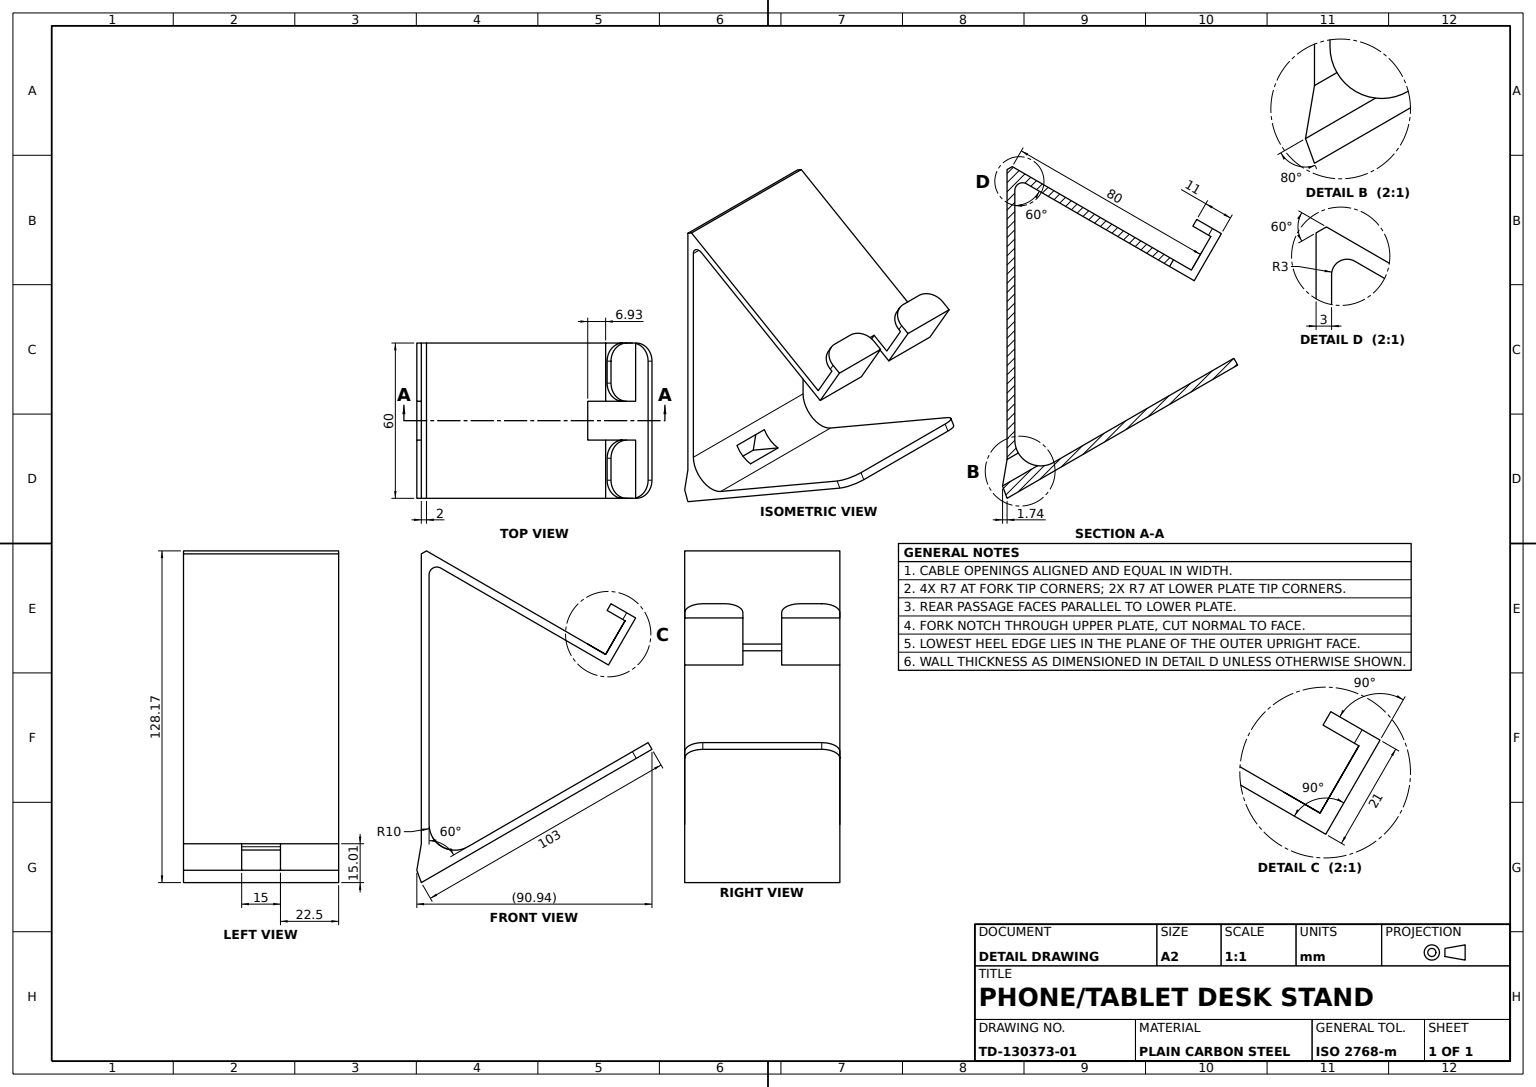
SolidWorks part; units mm, degrees
material "Plain Carbon Steel"
ref_plane "Front Plane" through (0, 0, 0) normal (0, 0, 1) x (1, 0, 0)
ref_plane "Top Plane" through (0, 0, 0) normal (0, 1, 0) x (1, 0, 0)
ref_plane "Right Plane" through (0, 0, 0) normal (1, 0, 0) x (0, 0, -1)
sketch "Stand Profile Sketch" plane through (0, 0, 0) normal (0, 0, 1) x (1, 0, 0)
  line L0 (0, 0) -> (80.4833, 0)
  line L1 (89.1436, 15) -> (40.9348, 98.5)
  line L2 (35.7387, 98.5) -> (-1.7199, 33.6199)
  line L3 (-1.7199, 33.6199) -> (-19.9064, 44.1199)
  line L4 (-19.9064, 44.1199) -> (-14.4064, 53.6462)
  line L5 (0, -3) -> (103, -3)
  line L6 (95.4944, 10) -> (39.4915, 107)
  line L7 (37.1821, 107) -> (-2.8179, 37.718)
  line L8 (-2.8179, 37.718) -> (-15.8083, 45.218)
  line L9 (-15.8083, 45.218) -> (-11.8083, 52.1462)
  line L10 (-14.4064, 53.6462) -> (-11.8083, 52.1462)
  line L11 (0, 0) -> (0, -3)
  line L12 (97.8038, 0) -> (95.4944, 10) construction
  line L13 (103, -3) -> (38.3368, 109) construction
  line L14 (103, -3) -> (102.1184, 2)
  line L15 (0, 0) -> (97.8038, 0) construction
  line L16 (97.8038, 0) -> (38.3368, 103) construction
  line L17 (95.4944, 10) -> (102.1184, 2)
  line L18 (38.3368, 103) -> (-1.7199, 33.6199) construction
  line L21 (37.1821, 107) -> (39.4915, 107)
  line L22 (38.3368, 109) -> (-2.8179, 37.718) construction
  arc A0 (80.4833, 0) -> (89.1436, 15) centre (80.4833, 10) ccw
  arc A2 (40.9348, 98.5) -> (35.7387, 98.5) centre (38.3368, 97) ccw
  point P17 (102.1184, 2)
  dimension "D9" = 10
  dimension "D13" = 35.7387
  dimension "D14" = 3
  dimension "D2" = 83
  dimension "D3" = 60
  dimension "D5" = 103
  dimension "D6" = 5
  dimension "D7" = 80
  dimension "D8" = 60
  dimension "D10" = 8
  dimension "D11" = 11
  dimension "D12" = 21
  dimension "D15" = 110
  dimension "D4" = 3
extrude "Stand Body 60mm" add sketch "Stand Profile Sketch" along normal mid plane 60
sketch "Cable Notch Sketch" plane through (0, 0, 0) normal (1, 0, 0) x (0, 0, -1)
  line L0 (-30, -3) -> (30, -3) construction
  line L1 (-7.5, 2) -> (7.5, 2)
  line L2 (-7.5, 2) -> (-7.5, 10)
  line L3 (-7.5, 10) -> (7.5, 10)
  line L4 (7.5, 2) -> (7.5, 10)
  line L5 (-7.5, 2) -> (7.5, 10) construction
  line L6 (-7.5, 10) -> (7.5, 2) construction
  point P0 (0, 6)
  dimension "D1" = 5
  dimension "D2" = 8
  dimension "D3" = 15
extrude "Cable Notch" cut sketch "Cable Notch Sketch" along normal through all
sketch "Slot 15x11 Sketch" plane through (-34.0343, 19.6497, 0) normal (-0.866, 0.5, 0) x (0, 0, 1)
  line L0 (30, 39.2558) -> (-30, 39.2558) construction
  line L1 (-7.5, 28.2558) -> (7.5, 28.2558)
  line L2 (-7.5, 28.2558) -> (-7.5, 39.2558)
  line L3 (-7.5, 39.2558) -> (7.5, 39.2558)
  line L4 (7.5, 28.2558) -> (7.5, 39.2558)
  line L5 (-7.5, 28.2558) -> (7.5, 39.2558) construction
  line L6 (-7.5, 39.2558) -> (7.5, 28.2558) construction
  point P0 (0, 33.7558)
  dimension "D1" = 15
  dimension "D2" = 11
extrude "Slot 15x11" cut sketch "Slot 15x11 Sketch" against normal up to next
fillet "Slot Edge Fillet R7" radius 7 4 edges at (-13.1073, 52.8962, 7.5) (-13.1073, 52.8962, 30) (-13.1073, 52.8962, -7.5) (-13.1073, 52.8962, -30)
fillet "Bend Fillet R7" radius 7 2 edges at (0, -1.5, -30) (0, -1.5, 30)
